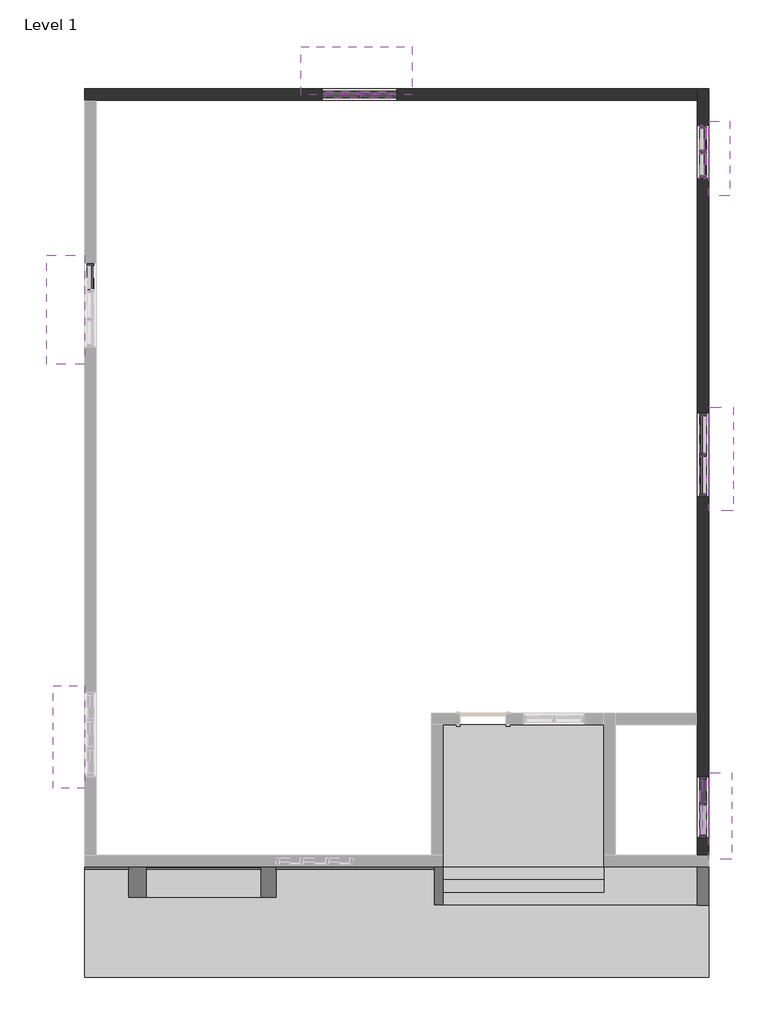
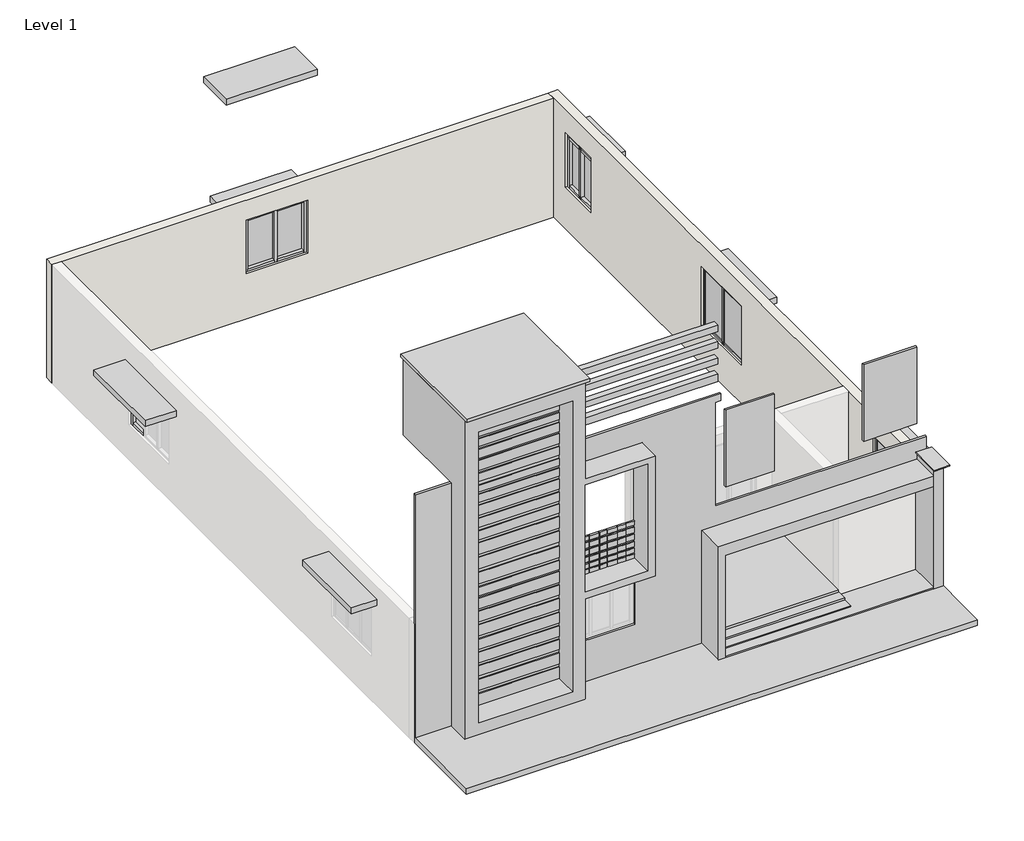
# One storey, part 2 of 2: 32 members, 10 plates, 10 proxies, 2 walls.
"""IFC4 building model written with IfcOpenShell, lengths in millimetres."""

from ifc_helpers import new_model, si_unit, origin, place, context, project, spatial, faceted_brep, transform, mapped, element, save
from components import generic_models_1_generic_models_1_34925b1c, generic_models_11_generic_models_11_b310268c, generic_models_12_generic_models_12_5e433632, generic_models_14_generic_models_14_0d0b8766, generic_models_2_generic_models_2_d48e4085, generic_models_3_generic_models_3_3f7da236, generic_models_5_generic_models_5_751a22c3, generic_models_6_generic_models_6_be8df775, generic_models_7_generic_models_7_8d3c1b96, generic_models_8_generic_models_8_3ed65b9d, member_6fb4a552, member_ad4059f0, member_4214a330, member_e5d39754, member_3a0a7659, member_32e692cc, member_44b7b902, member_7190e7de, member_505fbe18, member_a8e3eee7, member_f10a135f, member_a1fdef72, member_5535eeb3, member_041bc147, member_5215b92c, member_388f8896, member_80f955c2, system_panel_glazed_f327d843, system_panel_glazed_947315be, system_panel_glazed_af7a4178, system_panel_glazed_19038302, system_panel_glazed_da88386f, system_panel_glazed_1f6aae05

model = new_model("IFC4")

# Units and contexts
model_context = context("Model", 3, world=origin())
ifc_project = project(units=[si_unit("LENGTHUNIT", "METRE", prefix="MILLI")], contexts=[model_context])

# Site, building, storey
site = spatial("IfcSite", under=ifc_project)
building = spatial("IfcBuilding", under=site)
storey = spatial("IfcBuildingStorey", under=building, Name="Level 1", Elevation=0.0)

# Proxies
placement = place(None, origin())
generic_models_1_generic_models_1_shape = generic_models_1_generic_models_1_34925b1c(model_context)
element("IfcBuildingElementProxy", 1, Name="Generic Models 1 : Generic Models 1", ObjectType="Generic Models 1 : Generic Models 1", at=placement, inside=storey, context=model_context, shape_type="MappedRepresentation", body=[
    mapped(generic_models_1_generic_models_1_shape, transform((0.0, 0.0, 0.0), x_axis=(1.0, 0.0, 0.0), y_axis=(0.0, 1.0, 0.0), z_axis=(0.0, 0.0, 1.0))),
])
generic_models_11_generic_models_11_shape = generic_models_11_generic_models_11_b310268c(model_context)
element("IfcBuildingElementProxy", 2, Name="Generic Models 11 : Generic Models 11", ObjectType="Generic Models 11 : Generic Models 11", at=placement, inside=storey, context=model_context, shape_type="MappedRepresentation", body=[
    mapped(generic_models_11_generic_models_11_shape, transform((0.0, 0.0, 0.0), x_axis=(1.0, 0.0, 0.0), y_axis=(0.0, 1.0, 0.0), z_axis=(0.0, 0.0, 1.0))),
])
generic_models_12_generic_models_12_shape = generic_models_12_generic_models_12_5e433632(model_context)
element("IfcBuildingElementProxy", 3, Name="Generic Models 12 : Generic Models 12", ObjectType="Generic Models 12 : Generic Models 12", at=placement, inside=storey, context=model_context, shape_type="MappedRepresentation", body=[
    mapped(generic_models_12_generic_models_12_shape, transform((0.0, 0.0, 0.0), x_axis=(1.0, 0.0, 0.0), y_axis=(0.0, 1.0, 0.0), z_axis=(0.0, 0.0, 1.0))),
])
generic_models_14_generic_models_14_shape = generic_models_14_generic_models_14_0d0b8766(model_context)
element("IfcBuildingElementProxy", 4, Name="Generic Models 14 : Generic Models 14", ObjectType="Generic Models 14 : Generic Models 14", at=placement, inside=storey, context=model_context, shape_type="MappedRepresentation", body=[
    mapped(generic_models_14_generic_models_14_shape, transform((0.0, 0.0, 0.0), x_axis=(1.0, 0.0, 0.0), y_axis=(0.0, 1.0, 0.0), z_axis=(0.0, 0.0, 1.0))),
])
generic_models_2_generic_models_2_shape = generic_models_2_generic_models_2_d48e4085(model_context)
element("IfcBuildingElementProxy", 5, Name="Generic Models 2 : Generic Models 2", ObjectType="Generic Models 2 : Generic Models 2", at=placement, inside=storey, context=model_context, shape_type="MappedRepresentation", body=[
    mapped(generic_models_2_generic_models_2_shape, transform((0.0, 0.0, 0.0), x_axis=(1.0, 0.0, 0.0), y_axis=(0.0, 1.0, 0.0), z_axis=(0.0, 0.0, 1.0))),
])
generic_models_3_generic_models_3_shape = generic_models_3_generic_models_3_3f7da236(model_context)
element("IfcBuildingElementProxy", 6, Name="Generic Models 3 : Generic Models 3", ObjectType="Generic Models 3 : Generic Models 3", at=placement, inside=storey, context=model_context, shape_type="MappedRepresentation", body=[
    mapped(generic_models_3_generic_models_3_shape, transform((0.0, 0.0, 0.0), x_axis=(1.0, 0.0, 0.0), y_axis=(0.0, 1.0, 0.0), z_axis=(0.0, 0.0, 1.0))),
])
generic_models_5_generic_models_5_shape = generic_models_5_generic_models_5_751a22c3(model_context)
element("IfcBuildingElementProxy", 7, Name="Generic Models 5 : Generic Models 5", ObjectType="Generic Models 5 : Generic Models 5", at=placement, inside=storey, context=model_context, shape_type="MappedRepresentation", body=[
    mapped(generic_models_5_generic_models_5_shape, transform((0.0, 0.0, 0.0), x_axis=(1.0, 0.0, 0.0), y_axis=(0.0, 1.0, 0.0), z_axis=(0.0, 0.0, 1.0))),
])
generic_models_6_generic_models_6_shape = generic_models_6_generic_models_6_be8df775(model_context)
element("IfcBuildingElementProxy", 8, Name="Generic Models 6 : Generic Models 6", ObjectType="Generic Models 6 : Generic Models 6", at=placement, inside=storey, context=model_context, shape_type="MappedRepresentation", body=[
    mapped(generic_models_6_generic_models_6_shape, transform((0.0, 0.0, 0.0), x_axis=(1.0, 0.0, 0.0), y_axis=(0.0, 1.0, 0.0), z_axis=(0.0, 0.0, 1.0))),
])
generic_models_7_generic_models_7_shape = generic_models_7_generic_models_7_8d3c1b96(model_context)
element("IfcBuildingElementProxy", 9, Name="Generic Models 7 : Generic Models 7", ObjectType="Generic Models 7 : Generic Models 7", at=placement, inside=storey, context=model_context, shape_type="MappedRepresentation", body=[
    mapped(generic_models_7_generic_models_7_shape, transform((0.0, 0.0, 0.0), x_axis=(1.0, 0.0, 0.0), y_axis=(0.0, 1.0, 0.0), z_axis=(0.0, 0.0, 1.0))),
])
generic_models_8_generic_models_8_shape = generic_models_8_generic_models_8_3ed65b9d(model_context)
element("IfcBuildingElementProxy", 10, Name="Generic Models 8 : Generic Models 8", ObjectType="Generic Models 8 : Generic Models 8", at=placement, inside=storey, context=model_context, shape_type="MappedRepresentation", body=[
    mapped(generic_models_8_generic_models_8_shape, transform((0.0, 0.0, 0.0), x_axis=(1.0, 0.0, 0.0), y_axis=(0.0, 1.0, 0.0), z_axis=(0.0, 0.0, 1.0))),
])

# Members
member_shape = member_6fb4a552(model_context)
element("IfcMember", 11, ObjectType="Rectangular Mullion : 2.5\" x 5\" rectangular", at=placement, inside=storey, context=model_context, shape_type="MappedRepresentation", body=[
    mapped(member_shape, transform((-3916.7859258, -10512.0277232, 1144.0804944), x_axis=(0.0, 0.0, -1.0), y_axis=(1.0, 0.0, 0.0), z_axis=(0.0, -1.0, 0.0))),
])
element("IfcMember", 12, ObjectType="Rectangular Mullion : 2.5\" x 5\" rectangular", at=placement, inside=storey, context=model_context, shape_type="MappedRepresentation", body=[
    mapped(member_shape, transform((-3916.7859258, 2378.4722768, 1063.0916382), x_axis=(0.0, 0.0, -1.0), y_axis=(-1.0, 0.0, 0.0), z_axis=(0.0, 1.0, 0.0))),
])
element("IfcMember", 13, ObjectType="Rectangular Mullion : 2.5\" x 5\" rectangular", at=placement, inside=storey, context=model_context, shape_type="MappedRepresentation", body=[
    mapped(member_shape, transform((-3916.7859258, 2880.1222768, 1063.0916382), x_axis=(0.0, 0.0, -1.0), y_axis=(-1.0, 0.0, 0.0), z_axis=(0.0, 1.0, 0.0))),
])
member_2_shape = member_ad4059f0(model_context)
element("IfcMember", 14, ObjectType="Rectangular Mullion : 2.5\" x 5\" rectangular", at=placement, inside=storey, context=model_context, shape_type="MappedRepresentation", body=[
    mapped(member_2_shape, transform((-3916.7859258, -10543.7777232, 1144.0804944), x_axis=(0.0, 1.0, 0.0), y_axis=(1.0, 0.0, 0.0), z_axis=(0.0, 0.0, -1.0))),
])
element("IfcMember", 15, ObjectType="Rectangular Mullion : 2.5\" x 5\" rectangular", at=placement, inside=storey, context=model_context, shape_type="MappedRepresentation", body=[
    mapped(member_shape, transform((-3916.7859258, -10073.8777232, 2520.0251482), x_axis=(0.0, 0.0, 1.0), y_axis=(1.0, 0.0, 0.0), z_axis=(0.0, 1.0, 0.0))),
])
member_3_shape = member_4214a330(model_context)
element("IfcMember", 16, ObjectType="Rectangular Mullion : 2.5\" x 5\" rectangular", at=placement, inside=storey, context=model_context, shape_type="MappedRepresentation", body=[
    mapped(member_3_shape, transform((-3916.7859258, -10010.3777232, 1144.0804944), x_axis=(0.0, 1.0, 0.0), y_axis=(1.0, 0.0, 0.0), z_axis=(0.0, 0.0, -1.0))),
])
member_4_shape = member_e5d39754(model_context)
element("IfcMember", 17, ObjectType="Rectangular Mullion : 2.5\" x 5\" rectangular", at=placement, inside=storey, context=model_context, shape_type="MappedRepresentation", body=[
    mapped(member_4_shape, transform((-3916.7859258, -10575.5277232, 2520.0251482), x_axis=(0.0, 0.0, 1.0), y_axis=(1.0, 0.0, 0.0), z_axis=(0.0, 1.0, 0.0))),
])
element("IfcMember", 18, ObjectType="Rectangular Mullion : 2.5\" x 5\" rectangular", at=placement, inside=storey, context=model_context, shape_type="MappedRepresentation", body=[
    mapped(member_3_shape, transform((-3916.7859258, -11229.5777232, 2520.0251482), x_axis=(0.0, -1.0, 0.0), y_axis=(1.0, 0.0, 0.0), z_axis=(0.0, 0.0, 1.0))),
])
member_5_shape = member_3a0a7659(model_context)
element("IfcMember", 19, ObjectType="Rectangular Mullion : 2.5\" x 5\" rectangular", at=placement, inside=storey, context=model_context, shape_type="MappedRepresentation", body=[
    mapped(member_5_shape, transform((-3916.7859258, -3577.8277232, 971.2264169), x_axis=(0.0, 0.0, -1.0), y_axis=(1.0, 0.0, 0.0), z_axis=(0.0, -1.0, 0.0))),
])
element("IfcMember", 20, ObjectType="Rectangular Mullion : 2.5\" x 5\" rectangular", at=placement, inside=storey, context=model_context, shape_type="MappedRepresentation", body=[
    mapped(member_5_shape, transform((-3916.7859258, -4384.2777232, 971.2264169), x_axis=(0.0, 0.0, -1.0), y_axis=(1.0, 0.0, 0.0), z_axis=(0.0, -1.0, 0.0))),
])
member_6_shape = member_32e692cc(model_context)
element("IfcMember", 21, ObjectType="Rectangular Mullion : 2.5\" x 5\" rectangular", at=placement, inside=storey, context=model_context, shape_type="MappedRepresentation", body=[
    mapped(member_6_shape, transform((-3916.7859258, -3609.5777232, 971.2264169), x_axis=(0.0, 1.0, 0.0), y_axis=(1.0, 0.0, 0.0), z_axis=(0.0, 0.0, -1.0))),
])
element("IfcMember", 22, ObjectType="Rectangular Mullion : 2.5\" x 5\" rectangular", at=placement, inside=storey, context=model_context, shape_type="MappedRepresentation", body=[
    mapped(member_5_shape, transform((-3916.7859258, -3641.3277232, 2487.6320874), x_axis=(0.0, 0.0, 1.0), y_axis=(1.0, 0.0, 0.0), z_axis=(0.0, 1.0, 0.0))),
])
element("IfcMember", 23, ObjectType="Rectangular Mullion : 2.5\" x 5\" rectangular", at=placement, inside=storey, context=model_context, shape_type="MappedRepresentation", body=[
    mapped(member_5_shape, transform((-3916.7859258, -2834.8777232, 2487.6320874), x_axis=(0.0, 0.0, 1.0), y_axis=(1.0, 0.0, 0.0), z_axis=(0.0, 1.0, 0.0))),
])
member_7_shape = member_44b7b902(model_context)
element("IfcMember", 24, ObjectType="Rectangular Mullion : 2.5\" x 5\" rectangular", at=placement, inside=storey, context=model_context, shape_type="MappedRepresentation", body=[
    mapped(member_7_shape, transform((-3916.7859258, -2771.3777232, 971.2264169), x_axis=(0.0, 1.0, 0.0), y_axis=(1.0, 0.0, 0.0), z_axis=(0.0, 0.0, -1.0))),
])
element("IfcMember", 25, ObjectType="Rectangular Mullion : 2.5\" x 5\" rectangular", at=placement, inside=storey, context=model_context, shape_type="MappedRepresentation", body=[
    mapped(member_7_shape, transform((-3916.7859258, -4447.7777232, 2487.6320874), x_axis=(0.0, -1.0, 0.0), y_axis=(1.0, 0.0, 0.0), z_axis=(0.0, 0.0, 1.0))),
])
member_8_shape = member_7190e7de(model_context)
element("IfcMember", 26, ObjectType="Rectangular Mullion : 2.5\" x 5\" rectangular", at=placement, inside=storey, context=model_context, shape_type="MappedRepresentation", body=[
    mapped(member_8_shape, transform((-3916.7859258, 2410.2222768, 2346.010234), x_axis=(0.0, -1.0, 0.0), y_axis=(-1.0, 0.0, 0.0), z_axis=(0.0, 0.0, -1.0))),
])
member_9_shape = member_505fbe18(model_context)
element("IfcMember", 27, ObjectType="Rectangular Mullion : 2.5\" x 5\" rectangular", at=placement, inside=storey, context=model_context, shape_type="MappedRepresentation", body=[
    mapped(member_9_shape, transform((-3916.7859258, 1940.3222768, 2346.010234), x_axis=(0.0, 0.0, 1.0), y_axis=(-1.0, 0.0, 0.0), z_axis=(0.0, -1.0, 0.0))),
])
element("IfcMember", 28, ObjectType="Rectangular Mullion : 2.5\" x 5\" rectangular", at=placement, inside=storey, context=model_context, shape_type="MappedRepresentation", body=[
    mapped(member_9_shape, transform((-3916.7859258, 2441.9722768, 2346.010234), x_axis=(0.0, 0.0, 1.0), y_axis=(-1.0, 0.0, 0.0), z_axis=(0.0, -1.0, 0.0))),
])
member_10_shape = member_a8e3eee7(model_context)
element("IfcMember", 29, ObjectType="Rectangular Mullion : 2.5\" x 5\" rectangular", at=placement, inside=storey, context=model_context, shape_type="MappedRepresentation", body=[
    mapped(member_10_shape, transform((-3916.7859258, 2943.6222768, 2473.010234), x_axis=(0.0, 1.0, 0.0), y_axis=(-1.0, 0.0, 0.0), z_axis=(0.0, 0.0, 1.0))),
])
member_11_shape = member_f10a135f(model_context)
element("IfcMember", 30, ObjectType="Rectangular Mullion : 2.5\" x 5\" rectangular", at=placement, inside=storey, context=model_context, shape_type="MappedRepresentation", body=[
    mapped(member_11_shape, transform((-3916.7859258, 2410.2222768, 1063.0916382), x_axis=(0.0, -1.0, 0.0), y_axis=(-1.0, 0.0, 0.0), z_axis=(0.0, 0.0, -1.0))),
])
member_12_shape = member_a1fdef72(model_context)
element("IfcMember", 31, ObjectType="Rectangular Mullion : 2.5\" x 5\" rectangular", at=placement, inside=storey, context=model_context, shape_type="MappedRepresentation", body=[
    mapped(member_12_shape, transform((-3916.7859258, 2943.6222768, 2346.010234), x_axis=(0.0, 1.0, 0.0), y_axis=(-1.0, 0.0, 0.0), z_axis=(0.0, 0.0, 1.0))),
])
element("IfcMember", 32, ObjectType="Rectangular Mullion : 2.5\" x 5\" rectangular", at=placement, inside=storey, context=model_context, shape_type="MappedRepresentation", body=[
    mapped(member_10_shape, transform((-3916.7859258, 1876.8222768, 2346.010234), x_axis=(0.0, -1.0, 0.0), y_axis=(-1.0, 0.0, 0.0), z_axis=(0.0, 0.0, -1.0))),
])
element("IfcMember", 33, ObjectType="Rectangular Mullion : 2.5\" x 5\" rectangular", at=placement, inside=storey, context=model_context, shape_type="MappedRepresentation", body=[
    mapped(member_12_shape, transform((-3916.7859258, 1876.8222768, 1063.0916382), x_axis=(0.0, -1.0, 0.0), y_axis=(-1.0, 0.0, 0.0), z_axis=(0.0, 0.0, -1.0))),
])
member_13_shape = member_5535eeb3(model_context)
element("IfcMember", 34, ObjectType="Rectangular Mullion : 2.5\" x 5\" rectangular", at=placement, inside=storey, context=model_context, shape_type="MappedRepresentation", body=[
    mapped(member_13_shape, transform((-16108.7859258, 136.9222768, 897.5231842), x_axis=(0.0, 0.0, -1.0), y_axis=(-1.0, 0.0, 0.0), z_axis=(0.0, 1.0, 0.0))),
])
member_14_shape = member_041bc147(model_context)
element("IfcMember", 35, ObjectType="Rectangular Mullion : 2.5\" x 5\" rectangular", at=placement, inside=storey, context=model_context, shape_type="MappedRepresentation", body=[
    mapped(member_14_shape, transform((-16108.7859258, 200.4222768, 2325.7757409), x_axis=(0.0, 1.0, 0.0), y_axis=(-1.0, 0.0, 0.0), z_axis=(0.0, 0.0, 1.0))),
])
member_15_shape = member_5215b92c(model_context)
element("IfcMember", 36, ObjectType="Rectangular Mullion : 2.5\" x 5\" rectangular", at=placement, inside=storey, context=model_context, shape_type="MappedRepresentation", body=[
    mapped(member_15_shape, transform((-10787.4859258, 3553.2222768, 2530.5665304), x_axis=(0.0, 0.0, 1.0), y_axis=(0.0, -1.0, 0.0), z_axis=(1.0, 0.0, 0.0))),
])
element("IfcMember", 37, ObjectType="Rectangular Mullion : 2.5\" x 5\" rectangular", at=placement, inside=storey, context=model_context, shape_type="MappedRepresentation", body=[
    mapped(member_15_shape, transform((-10076.2859258, 3553.2222768, 2530.5665304), x_axis=(0.0, 0.0, 1.0), y_axis=(0.0, -1.0, 0.0), z_axis=(1.0, 0.0, 0.0))),
])
element("IfcMember", 38, ObjectType="Rectangular Mullion : 2.5\" x 5\" rectangular", at=placement, inside=storey, context=model_context, shape_type="MappedRepresentation", body=[
    mapped(member_15_shape, transform((-10723.9859258, 3553.2222768, 1164.2530754), x_axis=(0.0, 0.0, -1.0), y_axis=(0.0, -1.0, 0.0), z_axis=(-1.0, 0.0, 0.0))),
])
element("IfcMember", 39, ObjectType="Rectangular Mullion : 2.5\" x 5\" rectangular", at=placement, inside=storey, context=model_context, shape_type="MappedRepresentation", body=[
    mapped(member_15_shape, transform((-11435.1859258, 3553.2222768, 1164.2530754), x_axis=(0.0, 0.0, -1.0), y_axis=(0.0, -1.0, 0.0), z_axis=(-1.0, 0.0, 0.0))),
])
member_16_shape = member_388f8896(model_context)
element("IfcMember", 40, ObjectType="Rectangular Mullion : 2.5\" x 5\" rectangular", at=placement, inside=storey, context=model_context, shape_type="MappedRepresentation", body=[
    mapped(member_16_shape, transform((-10755.7359258, 3553.2222768, 1164.2530754), x_axis=(1.0, 0.0, 0.0), y_axis=(0.0, -1.0, 0.0), z_axis=(0.0, 0.0, -1.0))),
])
member_17_shape = member_80f955c2(model_context)
element("IfcMember", 41, ObjectType="Rectangular Mullion : 2.5\" x 5\" rectangular", at=placement, inside=storey, context=model_context, shape_type="MappedRepresentation", body=[
    mapped(member_17_shape, transform((-10012.7859258, 3553.2222768, 1164.2530754), x_axis=(1.0, 0.0, 0.0), y_axis=(0.0, -1.0, 0.0), z_axis=(0.0, 0.0, -1.0))),
])
element("IfcMember", 42, ObjectType="Rectangular Mullion : 2.5\" x 5\" rectangular", at=placement, inside=storey, context=model_context, shape_type="MappedRepresentation", body=[
    mapped(member_17_shape, transform((-11498.6859258, 3553.2222768, 2530.5665304), x_axis=(-1.0, 0.0, 0.0), y_axis=(0.0, -1.0, 0.0), z_axis=(0.0, 0.0, 1.0))),
])

# Plates
system_panel_glazed_shape = system_panel_glazed_f327d843(model_context)
element("IfcPlate", 43, ObjectType="System Panel : Glazed", at=placement, inside=storey, context=model_context, shape_type="MappedRepresentation", body=[
    mapped(system_panel_glazed_shape, transform((-3916.7859258, -10292.9527232, 1207.5804944), x_axis=(0.0, 1.0, 0.0), y_axis=(-1.0, 0.0, 0.0), z_axis=(0.0, 0.0, 1.0))),
])
system_panel_glazed_2_shape = system_panel_glazed_947315be(model_context)
element("IfcPlate", 44, ObjectType="System Panel : Glazed", at=placement, inside=storey, context=model_context, shape_type="MappedRepresentation", body=[
    mapped(system_panel_glazed_2_shape, transform((-3916.7859258, -10870.8027232, 1207.5804944), x_axis=(0.0, 1.0, 0.0), y_axis=(-1.0, 0.0, 0.0), z_axis=(0.0, 0.0, 1.0))),
])
system_panel_glazed_3_shape = system_panel_glazed_af7a4178(model_context)
element("IfcPlate", 45, ObjectType="System Panel : Glazed", at=placement, inside=storey, context=model_context, shape_type="MappedRepresentation", body=[
    mapped(system_panel_glazed_3_shape, transform((-3916.7859258, -4012.8027232, 1034.7264169), x_axis=(0.0, 1.0, 0.0), y_axis=(-1.0, 0.0, 0.0), z_axis=(0.0, 0.0, 1.0))),
])
element("IfcPlate", 46, ObjectType="System Panel : Glazed", at=placement, inside=storey, context=model_context, shape_type="MappedRepresentation", body=[
    mapped(system_panel_glazed_3_shape, transform((-3916.7859258, -3206.3527232, 1034.7264169), x_axis=(0.0, 1.0, 0.0), y_axis=(-1.0, 0.0, 0.0), z_axis=(0.0, 0.0, 1.0))),
])
system_panel_glazed_4_shape = system_panel_glazed_19038302(model_context)
element("IfcPlate", 47, ObjectType="System Panel : Glazed", at=placement, inside=storey, context=model_context, shape_type="MappedRepresentation", body=[
    mapped(system_panel_glazed_4_shape, transform((-3916.7859258, 2661.0472768, 2377.760234), x_axis=(0.0, -1.0, 0.0), y_axis=(1.0, 0.0, 0.0), z_axis=(0.0, 0.0, 1.0))),
])
element("IfcPlate", 48, ObjectType="System Panel : Glazed", at=placement, inside=storey, context=model_context, shape_type="MappedRepresentation", body=[
    mapped(system_panel_glazed_4_shape, transform((-3916.7859258, 2159.3972768, 2377.760234), x_axis=(0.0, -1.0, 0.0), y_axis=(1.0, 0.0, 0.0), z_axis=(0.0, 0.0, 1.0))),
])
system_panel_glazed_5_shape = system_panel_glazed_da88386f(model_context)
element("IfcPlate", 49, ObjectType="System Panel : Glazed", at=placement, inside=storey, context=model_context, shape_type="MappedRepresentation", body=[
    mapped(system_panel_glazed_5_shape, transform((-3916.7859258, 2661.0472768, 1126.5916382), x_axis=(0.0, -1.0, 0.0), y_axis=(1.0, 0.0, 0.0), z_axis=(0.0, 0.0, 1.0))),
])
element("IfcPlate", 50, ObjectType="System Panel : Glazed", at=placement, inside=storey, context=model_context, shape_type="MappedRepresentation", body=[
    mapped(system_panel_glazed_5_shape, transform((-3916.7859258, 2159.3972768, 1126.5916382), x_axis=(0.0, -1.0, 0.0), y_axis=(1.0, 0.0, 0.0), z_axis=(0.0, 0.0, 1.0))),
])
system_panel_glazed_6_shape = system_panel_glazed_1f6aae05(model_context)
element("IfcPlate", 51, ObjectType="System Panel : Glazed", at=placement, inside=storey, context=model_context, shape_type="MappedRepresentation", body=[
    mapped(system_panel_glazed_6_shape, transform((-11111.3359258, 3553.2222768, 1227.7530754), x_axis=(1.0, 0.0, 0.0), y_axis=(0.0, 1.0, 0.0), z_axis=(0.0, 0.0, 1.0))),
])
element("IfcPlate", 52, ObjectType="System Panel : Glazed", at=placement, inside=storey, context=model_context, shape_type="MappedRepresentation", body=[
    mapped(system_panel_glazed_6_shape, transform((-10400.1359258, 3553.2222768, 1227.7530754), x_axis=(1.0, 0.0, 0.0), y_axis=(0.0, 1.0, 0.0), z_axis=(0.0, 0.0, 1.0))),
])

# Walls
element("IfcWall", 53, ObjectType="9\"", at=placement, inside=storey, context=model_context, shape_type="Brep", body=[
    faceted_brep([(-3802.4859258, -11572.4777232, 0.0), (-3802.4859258, 3667.5222768, 0.0), (-3802.4859258, 3667.5222768, 3048.0), (-3802.4859258, -11572.4777232, 3048.0), (-3802.4859258, -11229.5777232, 1144.0804944), (-3802.4859258, -11229.5777232, 2520.0251482), (-3802.4859258, -10010.3777232, 2520.0251482), (-3802.4859258, -10010.3777232, 1144.0804944), (-3802.4859258, -4447.7777232, 971.2264169), (-3802.4859258, -4447.7777232, 2487.6320874), (-3802.4859258, -2771.3777232, 2487.6320874), (-3802.4859258, -2771.3777232, 971.2264169), (-3802.4859258, 2943.6222768, 2473.010234), (-3802.4859258, 2943.6222768, 1063.0916382), (-3802.4859258, 1876.8222768, 1063.0916382), (-3802.4859258, 1876.8222768, 2473.010234), (-4031.0859258, 3667.5222768, 0.0), (-4031.0859258, 3438.9222768, 0.0), (-4031.0859258, -8753.0777232, 0.0), (-4031.0859258, -8981.6777232, 0.0), (-4031.0859258, -11572.4777232, 0.0), (-4031.0859258, -11572.4777232, 3048.0), (-4031.0859258, -8981.6777232, 3048.0), (-4031.0859258, -8753.0777232, 3048.0), (-4031.0859258, 3438.9222768, 3048.0), (-4031.0859258, 3667.5222768, 3048.0), (-4031.0859258, -11229.5777232, 2520.0251482), (-4031.0859258, -11229.5777232, 1144.0804944), (-4031.0859258, -10010.3777232, 1144.0804944), (-4031.0859258, -10010.3777232, 2520.0251482), (-4031.0859258, -4447.7777232, 2487.6320874), (-4031.0859258, -4447.7777232, 971.2264169), (-4031.0859258, -2771.3777232, 971.2264169), (-4031.0859258, -2771.3777232, 2487.6320874), (-4031.0859258, 2943.6222768, 1063.0916382), (-4031.0859258, 2943.6222768, 2473.010234), (-4031.0859258, 1876.8222768, 2473.010234), (-4031.0859258, 1876.8222768, 1063.0916382)], [[[0, 1, 2, 3], [4, 5, 6, 7], [8, 9, 10, 11], [12, 13, 14, 15]], [[16, 17, 18, 19, 20, 21, 22, 23, 24, 25], [26, 27, 28, 29], [30, 31, 32, 33], [34, 35, 36, 37]], [[1, 0, 20, 19, 18, 17, 16]], [[3, 2, 25, 24, 23, 22, 21]], [[0, 3, 21, 20]], [[2, 1, 16, 25]], [[4, 27, 26, 5]], [[5, 26, 29, 6]], [[6, 29, 28, 7]], [[27, 4, 7, 28]], [[30, 9, 8, 31]], [[9, 30, 33, 10]], [[10, 33, 32, 11]], [[31, 8, 11, 32]], [[34, 13, 12, 35]], [[35, 12, 15, 36]], [[14, 37, 36, 15]], [[13, 34, 37, 14]]]),
])
element("IfcWall", 54, ObjectType="9\"", at=placement, inside=storey, context=model_context, shape_type="Brep", body=[
    faceted_brep([(-4031.0859258, 3667.5222768, 0.0), (-16223.0859258, 3667.5222768, 0.0), (-16223.0859258, 3667.5222768, 3048.0), (-4031.0859258, 3667.5222768, 3048.0), (-11498.6859258, 3667.5222768, 2530.5665304), (-11498.6859258, 3667.5222768, 1164.2530754), (-10012.7859258, 3667.5222768, 1164.2530754), (-10012.7859258, 3667.5222768, 2530.5665304), (-16223.0859258, 3438.9222768, 0.0), (-15994.4859258, 3438.9222768, 0.0), (-4031.0859258, 3438.9222768, 0.0), (-4031.0859258, 3438.9222768, 3048.0), (-15994.4859258, 3438.9222768, 3048.0), (-16223.0859258, 3438.9222768, 3048.0), (-11498.6859258, 3438.9222768, 1164.2530754), (-11498.6859258, 3438.9222768, 2530.5665304), (-10012.7859258, 3438.9222768, 2530.5665304), (-10012.7859258, 3438.9222768, 1164.2530754)], [[[0, 1, 2, 3], [4, 5, 6, 7]], [[8, 9, 10, 11, 12, 13], [14, 15, 16, 17]], [[1, 0, 10, 9, 8]], [[3, 2, 13, 12, 11]], [[0, 3, 11, 10]], [[2, 1, 8, 13]], [[14, 5, 4, 15]], [[15, 4, 7, 16]], [[16, 7, 6, 17]], [[5, 14, 17, 6]]]),
])

save(model, "model.ifc")

# Revit data of these elements
# Type "Rectangular Mullion : 2.5\" x 5\" rectangular"
#   built-in parameter 1007304 = 0.416667 (stored number, unit not read)
#   built-in parameter 1007301 = 0.104167 (stored number, unit not read)
#   built-in parameter 1007300 = 0.104167 (stored number, unit not read)
# Type "System Panel : Glazed"
#   Construction Type Id = "GSP4R"
#   Analytic Construction = "1/8 in Pilkington single glazing"
#   Visual Light Transmittance = 0.9
#   Solar Heat Gain Coefficient = 0.86
#   Heat Transfer Coefficient (U) = 1.18115 BTU/(h·ft²·°F)
#   Define Thermal Properties by = 1
# Type "9\""
#   Assembly Code = "B2010"
#   Layers, outside or top first: 0' - 9" no material (function 1)
# Element 1 (IfcBuildingElementProxy, "Generic Models 1 : Generic Models 1")
#   Phase Created = New Construction
# Element 2 (IfcBuildingElementProxy, "Generic Models 11 : Generic Models 11")
#   Phase Created = New Construction
# Element 3 (IfcBuildingElementProxy, "Generic Models 12 : Generic Models 12")
#   Phase Created = New Construction
# Element 4 (IfcBuildingElementProxy, "Generic Models 14 : Generic Models 14")
#   Phase Created = New Construction
# Element 5 (IfcBuildingElementProxy, "Generic Models 2 : Generic Models 2")
#   Phase Created = New Construction
# Element 6 (IfcBuildingElementProxy, "Generic Models 3 : Generic Models 3")
#   Phase Created = New Construction
# Element 7 (IfcBuildingElementProxy, "Generic Models 5 : Generic Models 5")
#   Phase Created = New Construction
# Element 8 (IfcBuildingElementProxy, "Generic Models 6 : Generic Models 6")
#   Phase Created = New Construction
# Element 9 (IfcBuildingElementProxy, "Generic Models 7 : Generic Models 7")
#   Phase Created = New Construction
# Element 10 (IfcBuildingElementProxy, "Generic Models 8 : Generic Models 8")
#   Phase Created = New Construction
# Elements 11, 12, 13, 14, 15, 16, 17, 18, 19, 20, 21, 22, 23, 24, 25, 26, 27, 28, 29, 30, 31, 32, 33, 34, 35, 36, 37, 38, 39, 40, 41, 42 (IfcMember, "Rectangular Mullion : 2.5\" x 5\" rectangular")
#   Phase Created = New Construction
#   Materials on its faces: "Aluminum"
# Elements 43, 44, 45, 46, 47, 48, 49, 50, 51, 52 (IfcPlate, "System Panel : Glazed")
#   Phase Created = New Construction
#   Materials on its faces: "Glass"
# Elements 53, 54 (IfcWall, "9\"")
#   Top Offset = 0' - 0"
#   Base Offset = 0' - 0"
#   Unconnected Height = 10' - 0"
#   wall height = 10' - 0"
#   Phase Created = New Construction
#   Base Constraint = Level 1
#   Materials on its faces: "Default Wall"
# Materials
#   "Aluminum": class "Metal", colour RGB 247 247 247, transparency 0, Description = "Aluminum 6061", Cost = 0
#   "Glass": class "Glass", colour RGB 0 128 192, transparency 0.75, Description = "Soda Lime Glass", Cost = 0
#   "Default Wall": colour RGB 128 128 128, transparency 0, Cost = 0
